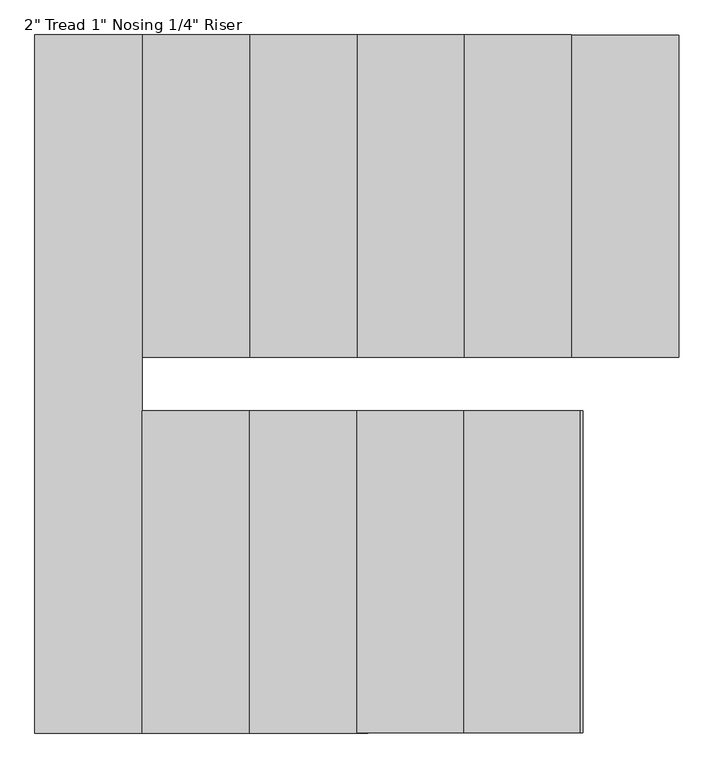
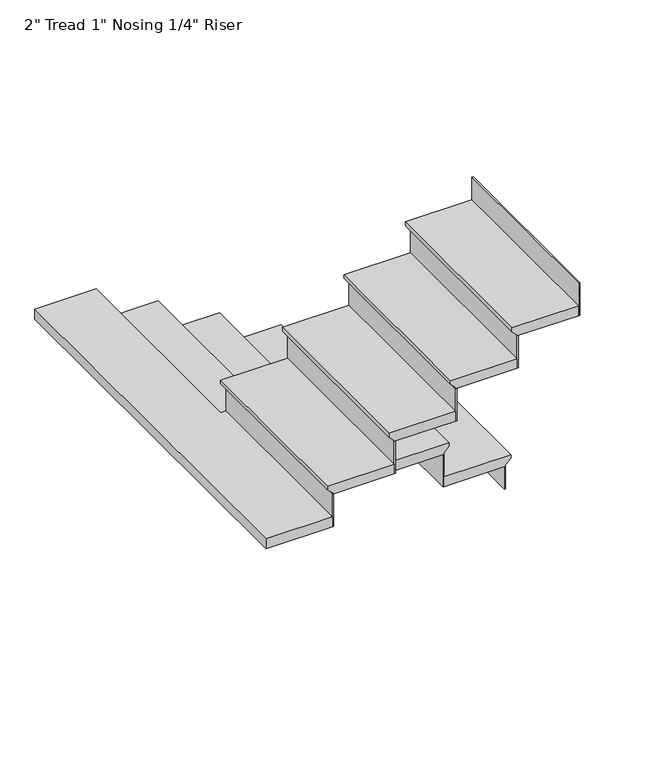
"""IFC4 building model written with IfcOpenShell, lengths in millimetres: stair flight geometry."""

from ifc_helpers import new_model, si_unit, origin, place, context, project, spatial, faceted_brep, source, transform, mapped, element, save


def stair_flight_da774960(model_context):
    return source(origin(), model_context, "Body", "Brep", [
        faceted_brep([(3327.4, 3340.1, 150.2833333), (3327.4, 3340.1, 169.3333333), (3327.4, 2425.7, 169.3333333), (3327.4, 2425.7, 150.2833333), (3302.0, 3340.1, 124.8833333), (3302.0, 2425.7, 124.8833333), (2997.2, 3340.1, 169.3333333), (2997.2, 2425.7, 169.3333333), (3302.0, 2425.7, 118.5333333), (2997.2, 2425.7, 118.5333333), (2997.2, 3340.1, 118.5333333), (3302.0, 3340.1, 118.5333333)], [[[0, 1, 2, 3]], [[4, 0, 3, 5]], [[2, 1, 6, 7]], [[8, 9, 10, 11]], [[2, 7, 9, 8, 5, 3]], [[8, 11, 4, 5]], [[6, 1, 0, 4, 11, 10]], [[7, 6, 10, 9]]]),
        faceted_brep([(3302.0, 3340.1, 118.5333333), (3302.0, 3340.1, 0.0), (3295.65, 3340.1, 0.0), (3295.65, 3340.1, 118.5333333), (3302.0, 2425.7, 118.5333333), (3295.65, 2425.7, 118.5333333), (3295.65, 2425.7, 0.0), (3302.0, 2425.7, 0.0)], [[[0, 1, 2, 3]], [[4, 5, 6, 7]], [[1, 0, 4, 7]], [[2, 1, 7, 6]], [[3, 2, 6, 5]], [[0, 3, 5, 4]]]),
        faceted_brep([(2997.2, 3340.1, 287.8666667), (2997.2, 3340.1, 118.5333333), (2990.85, 3340.1, 118.5333333), (2990.85, 3340.1, 287.8666667), (2997.2, 2425.7, 287.8666667), (2990.85, 2425.7, 287.8666667), (2990.85, 2425.7, 118.5333333), (2997.2, 2425.7, 118.5333333)], [[[0, 1, 2, 3]], [[4, 5, 6, 7]], [[1, 0, 4, 7]], [[2, 1, 7, 6]], [[3, 2, 6, 5]], [[0, 3, 5, 4]]]),
        faceted_brep([(3022.6, 2425.7, 338.6666667), (3022.6, 3340.1, 338.6666667), (2692.4, 3340.1, 338.6666667), (2692.4, 2425.7, 338.6666667), (2997.2, 2425.7, 287.8666667), (2692.4, 2425.7, 287.8666667), (2692.4, 3340.1, 287.8666667), (2997.2, 3340.1, 287.8666667), (2997.2, 2425.7, 294.2166667), (3022.6, 2425.7, 319.6166667), (2997.2, 3340.1, 294.2166667), (3022.6, 3340.1, 319.6166667)], [[[0, 1, 2, 3]], [[4, 5, 6, 7]], [[0, 3, 5, 4, 8, 9]], [[4, 7, 10, 8]], [[2, 1, 11, 10, 7, 6]], [[3, 2, 6, 5]], [[11, 1, 0, 9]], [[10, 11, 9, 8]]]),
        faceted_brep([(2692.4, 3340.1, 457.2), (2692.4, 3340.1, 287.8666667), (2686.05, 3340.1, 287.8666667), (2686.05, 3340.1, 457.2), (2692.4, 2425.7, 457.2), (2686.05, 2425.7, 457.2), (2686.05, 2425.7, 287.8666667), (2692.4, 2425.7, 287.8666667)], [[[0, 1, 2, 3]], [[4, 5, 6, 7]], [[1, 0, 4, 7]], [[2, 1, 7, 6]], [[3, 2, 6, 5]], [[0, 3, 5, 4]]]),
        faceted_brep([(2717.8, 2425.7, 508.0), (2717.8, 3340.1, 508.0), (2387.6, 3340.1, 508.0), (2387.6, 2425.7, 508.0), (2692.4, 2425.7, 457.2), (2387.6, 2425.7, 457.2), (2387.6, 3340.1, 457.2), (2692.4, 3340.1, 457.2), (2692.4, 2425.7, 463.55), (2717.8, 2425.7, 488.95), (2692.4, 3340.1, 463.55), (2717.8, 3340.1, 488.95)], [[[0, 1, 2, 3]], [[4, 5, 6, 7]], [[0, 3, 5, 4, 8, 9]], [[4, 7, 10, 8]], [[2, 1, 11, 10, 7, 6]], [[3, 2, 6, 5]], [[11, 1, 0, 9]], [[10, 11, 9, 8]]]),
        faceted_brep([(2387.6, 3340.1, 626.5333333), (2387.6, 3340.1, 457.2), (2381.25, 3340.1, 457.2), (2381.25, 3340.1, 626.5333333), (2387.6, 2425.7, 626.5333333), (2381.25, 2425.7, 626.5333333), (2381.25, 2425.7, 457.2), (2387.6, 2425.7, 457.2)], [[[0, 1, 2, 3]], [[4, 5, 6, 7]], [[1, 0, 4, 7]], [[2, 1, 7, 6]], [[3, 2, 6, 5]], [[0, 3, 5, 4]]]),
        faceted_brep([(2413.0, 2425.7, 677.3333333), (2413.0, 3340.1, 677.3333333), (2082.8, 3340.1, 677.3333333), (2082.8, 2425.7, 677.3333333), (2387.6, 2425.7, 626.5333333), (2082.8, 2425.7, 626.5333333), (2082.8, 3340.1, 626.5333333), (2387.6, 3340.1, 626.5333333), (2387.6, 2425.7, 632.8833333), (2413.0, 2425.7, 658.2833333), (2387.6, 3340.1, 632.8833333), (2413.0, 3340.1, 658.2833333)], [[[0, 1, 2, 3]], [[4, 5, 6, 7]], [[0, 3, 5, 4, 8, 9]], [[4, 7, 10, 8]], [[2, 1, 11, 10, 7, 6]], [[3, 2, 6, 5]], [[11, 1, 0, 9]], [[10, 11, 9, 8]]]),
        faceted_brep([(2082.8, 3340.1, 795.8666667), (2082.8, 3340.1, 626.5333333), (2076.45, 3340.1, 626.5333333), (2076.45, 3340.1, 795.8666667), (2082.8, 2425.7, 795.8666667), (2076.45, 2425.7, 795.8666667), (2076.45, 2425.7, 626.5333333), (2082.8, 2425.7, 626.5333333)], [[[0, 1, 2, 3]], [[4, 5, 6, 7]], [[1, 0, 4, 7]], [[2, 1, 7, 6]], [[3, 2, 6, 5]], [[0, 3, 5, 4]]]),
        faceted_brep([(2108.2, 2425.7, 846.6666667), (2108.2, 3340.1, 846.6666667), (1778.0, 3340.1, 846.6666667), (1778.0, 2425.7, 846.6666667), (2082.8, 2425.7, 795.8666667), (1778.0, 2425.7, 795.8666667), (1778.0, 3340.1, 795.8666667), (2082.8, 3340.1, 795.8666667), (2082.8, 2425.7, 802.2166667), (2108.2, 2425.7, 827.6166667), (2082.8, 3340.1, 802.2166667), (2108.2, 3340.1, 827.6166667)], [[[0, 1, 2, 3]], [[4, 5, 6, 7]], [[0, 3, 5, 4, 8, 9]], [[4, 7, 10, 8]], [[2, 1, 11, 10, 7, 6]], [[3, 2, 6, 5]], [[11, 1, 0, 9]], [[10, 11, 9, 8]]]),
        faceted_brep([(1778.0, 3340.1, 965.2), (1778.0, 3340.1, 795.8666667), (1771.65, 3340.1, 795.8666667), (1771.65, 3340.1, 965.2), (1778.0, 2425.7, 965.2), (1771.65, 2425.7, 965.2), (1771.65, 2425.7, 795.8666667), (1778.0, 2425.7, 795.8666667)], [[[0, 1, 2, 3]], [[4, 5, 6, 7]], [[1, 0, 4, 7]], [[2, 1, 7, 6]], [[3, 2, 6, 5]], [[0, 3, 5, 4]]]),
        faceted_brep([(1828.8, 2273.3, 1016.0), (1803.4, 2273.3, 1016.0), (1803.4, 3340.1, 1016.0), (1498.6, 3340.1, 1016.0), (1498.6, 1358.9, 1016.0), (1828.8, 1358.9, 1016.0), (1803.4, 2273.3, 965.2), (1828.8, 2273.3, 965.2), (1828.8, 1358.9, 965.2), (1498.6, 1358.9, 965.2), (1498.6, 3340.1, 965.2), (1778.0, 3340.1, 965.2), (1778.0, 2425.7, 965.2), (1803.4, 2425.7, 965.2), (1803.4, 2425.7, 996.95), (1803.4, 3340.1, 996.95), (1778.0, 2425.7, 971.55), (1778.0, 3340.1, 971.55)], [[[0, 1, 2, 3, 4, 5]], [[6, 7, 8, 9, 10, 11, 12, 13]], [[1, 0, 7, 6]], [[2, 1, 6, 13, 14, 15]], [[13, 12, 16, 14]], [[12, 11, 17, 16]], [[3, 2, 15, 17, 11, 10]], [[4, 3, 10, 9]], [[5, 4, 9, 8]], [[0, 5, 8, 7]], [[17, 15, 14, 16]]]),
        faceted_brep([(1828.8, 1358.9, 1134.5333333), (1828.8, 1358.9, 965.2), (1835.15, 1358.9, 965.2), (1835.15, 1358.9, 1134.5333333), (1828.8, 2273.3, 1134.5333333), (1835.15, 2273.3, 1134.5333333), (1835.15, 2273.3, 965.2), (1828.8, 2273.3, 965.2)], [[[0, 1, 2, 3]], [[4, 5, 6, 7]], [[1, 0, 4, 7]], [[2, 1, 7, 6]], [[3, 2, 6, 5]], [[0, 3, 5, 4]]]),
        faceted_brep([(1803.4, 2273.3, 1185.3333333), (1803.4, 1358.9, 1185.3333333), (2133.6, 1358.9, 1185.3333333), (2133.6, 2273.3, 1185.3333333), (1828.8, 2273.3, 1134.5333333), (2133.6, 2273.3, 1134.5333333), (2133.6, 1358.9, 1134.5333333), (1828.8, 1358.9, 1134.5333333), (1828.8, 2273.3, 1140.8833333), (1803.4, 2273.3, 1166.2833333), (1828.8, 1358.9, 1140.8833333), (1803.4, 1358.9, 1166.2833333)], [[[0, 1, 2, 3]], [[4, 5, 6, 7]], [[0, 3, 5, 4, 8, 9]], [[4, 7, 10, 8]], [[2, 1, 11, 10, 7, 6]], [[3, 2, 6, 5]], [[11, 1, 0, 9]], [[10, 11, 9, 8]]]),
        faceted_brep([(2133.6, 1358.9, 1303.8666667), (2133.6, 1358.9, 1134.5333333), (2139.95, 1358.9, 1134.5333333), (2139.95, 1358.9, 1303.8666667), (2133.6, 2273.3, 1303.8666667), (2139.95, 2273.3, 1303.8666667), (2139.95, 2273.3, 1134.5333333), (2133.6, 2273.3, 1134.5333333)], [[[0, 1, 2, 3]], [[4, 5, 6, 7]], [[1, 0, 4, 7]], [[2, 1, 7, 6]], [[3, 2, 6, 5]], [[0, 3, 5, 4]]]),
        faceted_brep([(2108.2, 2273.3, 1354.6666667), (2108.2, 1358.9, 1354.6666667), (2438.4, 1358.9, 1354.6666667), (2438.4, 2273.3, 1354.6666667), (2133.6, 2273.3, 1303.8666667), (2438.4, 2273.3, 1303.8666667), (2438.4, 1358.9, 1303.8666667), (2133.6, 1358.9, 1303.8666667), (2133.6, 2273.3, 1310.2166667), (2108.2, 2273.3, 1335.6166667), (2133.6, 1358.9, 1310.2166667), (2108.2, 1358.9, 1335.6166667)], [[[0, 1, 2, 3]], [[4, 5, 6, 7]], [[0, 3, 5, 4, 8, 9]], [[4, 7, 10, 8]], [[2, 1, 11, 10, 7, 6]], [[3, 2, 6, 5]], [[11, 1, 0, 9]], [[10, 11, 9, 8]]]),
        faceted_brep([(2438.4, 1358.9, 1473.2), (2438.4, 1358.9, 1303.8666667), (2444.75, 1358.9, 1303.8666667), (2444.75, 1358.9, 1473.2), (2438.4, 2273.3, 1473.2), (2444.75, 2273.3, 1473.2), (2444.75, 2273.3, 1303.8666667), (2438.4, 2273.3, 1303.8666667)], [[[0, 1, 2, 3]], [[4, 5, 6, 7]], [[1, 0, 4, 7]], [[2, 1, 7, 6]], [[3, 2, 6, 5]], [[0, 3, 5, 4]]]),
        faceted_brep([(2413.0, 2273.3, 1524.0), (2413.0, 1358.9, 1524.0), (2743.2, 1358.9, 1524.0), (2743.2, 2273.3, 1524.0), (2438.4, 2273.3, 1473.2), (2743.2, 2273.3, 1473.2), (2743.2, 1358.9, 1473.2), (2438.4, 1358.9, 1473.2), (2438.4, 2273.3, 1479.55), (2413.0, 2273.3, 1504.95), (2438.4, 1358.9, 1479.55), (2413.0, 1358.9, 1504.95)], [[[0, 1, 2, 3]], [[4, 5, 6, 7]], [[0, 3, 5, 4, 8, 9]], [[4, 7, 10, 8]], [[2, 1, 11, 10, 7, 6]], [[3, 2, 6, 5]], [[11, 1, 0, 9]], [[10, 11, 9, 8]]]),
        faceted_brep([(2743.2, 1358.9, 1642.5333333), (2743.2, 1358.9, 1473.2), (2749.55, 1358.9, 1473.2), (2749.55, 1358.9, 1642.5333333), (2743.2, 2273.3, 1642.5333333), (2749.55, 2273.3, 1642.5333333), (2749.55, 2273.3, 1473.2), (2743.2, 2273.3, 1473.2)], [[[0, 1, 2, 3]], [[4, 5, 6, 7]], [[1, 0, 4, 7]], [[2, 1, 7, 6]], [[3, 2, 6, 5]], [[0, 3, 5, 4]]]),
        faceted_brep([(3048.0, 1358.9, 1811.8666667), (3048.0, 1358.9, 1642.5333333), (3054.35, 1358.9, 1642.5333333), (3054.35, 1358.9, 1811.8666667), (3048.0, 2273.3, 1811.8666667), (3054.35, 2273.3, 1811.8666667), (3054.35, 2273.3, 1642.5333333), (3048.0, 2273.3, 1642.5333333)], [[[0, 1, 2, 3]], [[4, 5, 6, 7]], [[1, 0, 4, 7]], [[2, 1, 7, 6]], [[3, 2, 6, 5]], [[0, 3, 5, 4]]]),
        faceted_brep([(2717.8, 2273.3, 1693.3333333), (2717.8, 1358.9, 1693.3333333), (3048.0, 1358.9, 1693.3333333), (3048.0, 2273.3, 1693.3333333), (2743.2, 2273.3, 1642.5333333), (3048.0, 2273.3, 1642.5333333), (3048.0, 1358.9, 1642.5333333), (2743.2, 1358.9, 1642.5333333), (2743.2, 2273.3, 1648.8833333), (2717.8, 2273.3, 1674.2833333), (2743.2, 1358.9, 1648.8833333), (2717.8, 1358.9, 1674.2833333)], [[[0, 1, 2, 3]], [[4, 5, 6, 7]], [[0, 3, 5, 4, 8, 9]], [[4, 7, 10, 8]], [[2, 1, 11, 10, 7, 6]], [[3, 2, 6, 5]], [[11, 1, 0, 9]], [[10, 11, 9, 8]]]),
    ])


if __name__ == "__main__":
    model = new_model("IFC4")
    model_context = context("Model", 3, world=origin())
    ifc_project = project(units=[si_unit("LENGTHUNIT", "METRE", prefix="MILLI")], contexts=[model_context])
    site = spatial("IfcSite", under=ifc_project)
    building = spatial("IfcBuilding", under=site)
    placement = place(None, origin())
    stair_flight_shape = stair_flight_da774960(model_context)
    element("IfcStairFlight", 1, ObjectType="2\" Tread 1\" Nosing 1/4\" Riser", at=placement, inside=building, context=model_context, shape_type="MappedRepresentation", body=[
        mapped(stair_flight_shape, transform((0.0, 0.0, 0.0), x_axis=(1.0, 0.0, 0.0), y_axis=(0.0, 1.0, 0.0), z_axis=(0.0, 0.0, 1.0))),
    ])
    save(model, "model.ifc")
